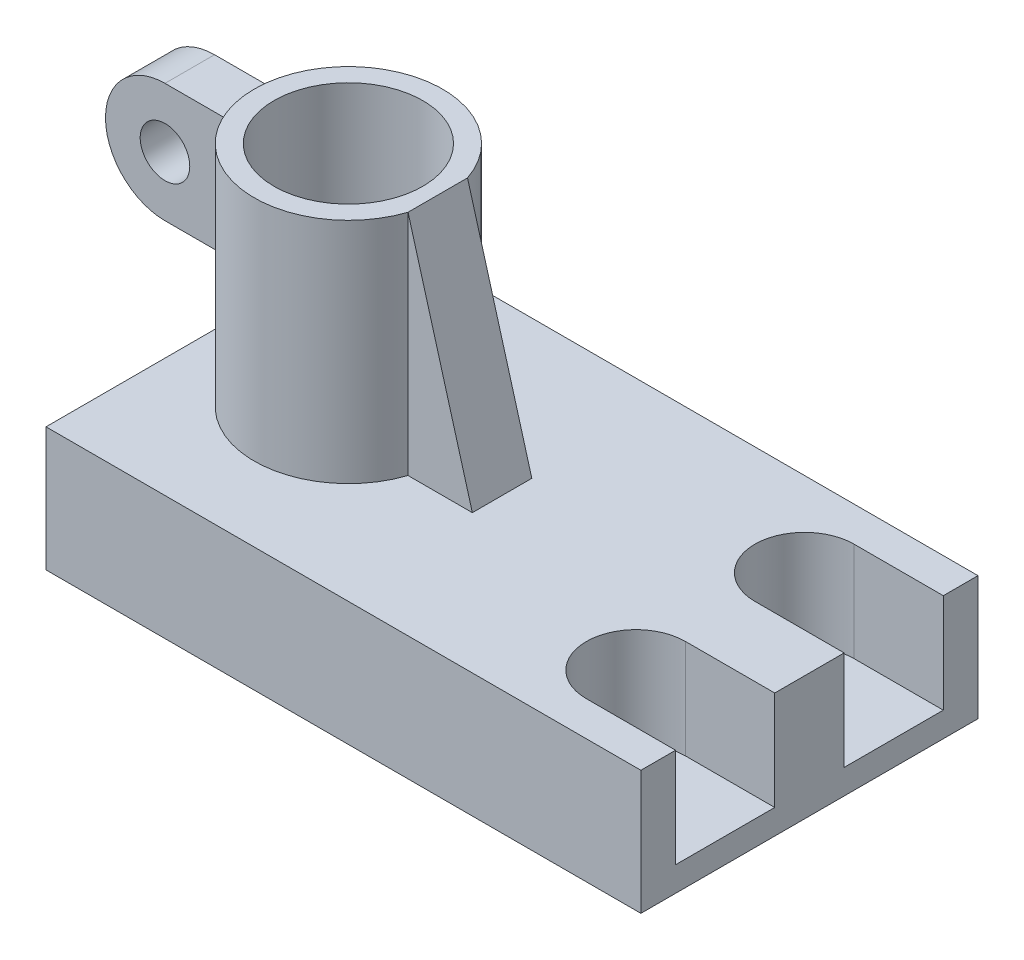
ISO-10303-21;
HEADER;
FILE_DESCRIPTION(('STEP AP214'),'2;1');
FILE_NAME('part.step','',(''),(''),'','','');
FILE_SCHEMA(('AUTOMOTIVE_DESIGN { 1 0 10303 214 1 1 1 1 }'));
ENDSEC;
DATA;
#1=APPLICATION_CONTEXT('core data for automotive mechanical design processes');
#2=APPLICATION_PROTOCOL_DEFINITION('international standard','automotive_design',2000,#1);
#3=PRODUCT_CONTEXT('',#1,'mechanical');
#4=PRODUCT('Part','Part','',(#3));
#5=PRODUCT_RELATED_PRODUCT_CATEGORY('part','',(#4));
#6=PRODUCT_DEFINITION_FORMATION('','',#4);
#7=PRODUCT_DEFINITION_CONTEXT('part definition',#1,'design');
#8=PRODUCT_DEFINITION('design','',#6,#7);
#9=PRODUCT_DEFINITION_SHAPE('','',#8);
#10=(LENGTH_UNIT() NAMED_UNIT(*) SI_UNIT(.MILLI.,.METRE.));
#11=(NAMED_UNIT(*) PLANE_ANGLE_UNIT() SI_UNIT($,.RADIAN.));
#12=(NAMED_UNIT(*) SI_UNIT($,.STERADIAN.) SOLID_ANGLE_UNIT());
#13=UNCERTAINTY_MEASURE_WITH_UNIT(LENGTH_MEASURE(1.E-05),#10,'distance_accuracy_value','');
#14=(GEOMETRIC_REPRESENTATION_CONTEXT(3) GLOBAL_UNCERTAINTY_ASSIGNED_CONTEXT((#13)) GLOBAL_UNIT_ASSIGNED_CONTEXT((#10,
#11,#12)) REPRESENTATION_CONTEXT('',''));
#15=CARTESIAN_POINT('',(0.,0.,0.));
#16=DIRECTION('',(0.,0.,1.));
#17=DIRECTION('',(1.,0.,0.));
#18=AXIS2_PLACEMENT_3D('',#15,#16,#17);
#19=CARTESIAN_POINT('',(60.,25.,34.));
#20=DIRECTION('',(-1.,0.,0.));
#21=DIRECTION('',(0.,0.,1.));
#22=AXIS2_PLACEMENT_3D('',#19,#20,#21);
#23=PLANE('',#22);
#24=DIRECTION('',(0.,0.,-1.));
#25=VECTOR('',#24,1.);
#26=CARTESIAN_POINT('',(60.,25.,34.));
#27=LINE('',#26,#25);
#28=CARTESIAN_POINT('',(60.,25.,7.));
#29=VERTEX_POINT('',#28);
#30=CARTESIAN_POINT('',(60.,25.,-7.));
#31=VERTEX_POINT('',#30);
#32=EDGE_CURVE('E216',#29,#31,#27,.T.);
#33=ORIENTED_EDGE('',*,*,#32,.F.);
#34=DIRECTION('',(0.,1.,0.));
#35=VECTOR('',#34,1.);
#36=CARTESIAN_POINT('',(60.,5.,7.));
#37=LINE('',#36,#35);
#38=CARTESIAN_POINT('',(60.,5.,7.));
#39=VERTEX_POINT('',#38);
#40=EDGE_CURVE('E329',#39,#29,#37,.T.);
#41=ORIENTED_EDGE('',*,*,#40,.F.);
#42=DIRECTION('',(0.,0.,-1.));
#43=VECTOR('',#42,1.);
#44=CARTESIAN_POINT('',(60.,5.,7.));
#45=LINE('',#44,#43);
#46=CARTESIAN_POINT('',(60.,5.,27.));
#47=VERTEX_POINT('',#46);
#48=EDGE_CURVE('E356',#47,#39,#45,.T.);
#49=ORIENTED_EDGE('',*,*,#48,.F.);
#50=DIRECTION('',(0.,1.,0.));
#51=VECTOR('',#50,1.);
#52=CARTESIAN_POINT('',(60.,5.,27.));
#53=LINE('',#52,#51);
#54=CARTESIAN_POINT('',(60.,25.,27.));
#55=VERTEX_POINT('',#54);
#56=EDGE_CURVE('E357',#47,#55,#53,.T.);
#57=ORIENTED_EDGE('',*,*,#56,.T.);
#58=CARTESIAN_POINT('',(60.,25.,34.));
#59=VERTEX_POINT('',#58);
#60=EDGE_CURVE('E213',#59,#55,#27,.T.);
#61=ORIENTED_EDGE('',*,*,#60,.F.);
#62=DIRECTION('',(0.,-1.,0.));
#63=VECTOR('',#62,1.);
#64=CARTESIAN_POINT('',(60.,25.,34.));
#65=LINE('',#64,#63);
#66=CARTESIAN_POINT('',(60.,0.,34.));
#67=VERTEX_POINT('',#66);
#68=EDGE_CURVE('E224',#59,#67,#65,.T.);
#69=ORIENTED_EDGE('',*,*,#68,.T.);
#70=DIRECTION('',(0.,0.,-1.));
#71=VECTOR('',#70,1.);
#72=CARTESIAN_POINT('',(60.,0.,34.));
#73=LINE('',#72,#71);
#74=CARTESIAN_POINT('',(60.,0.,-34.));
#75=VERTEX_POINT('',#74);
#76=EDGE_CURVE('E202',#67,#75,#73,.T.);
#77=ORIENTED_EDGE('',*,*,#76,.T.);
#78=DIRECTION('',(0.,-1.,0.));
#79=VECTOR('',#78,1.);
#80=CARTESIAN_POINT('',(60.,25.,-34.));
#81=LINE('',#80,#79);
#82=CARTESIAN_POINT('',(60.,25.,-34.));
#83=VERTEX_POINT('',#82);
#84=EDGE_CURVE('E239',#83,#75,#81,.T.);
#85=ORIENTED_EDGE('',*,*,#84,.F.);
#86=CARTESIAN_POINT('',(60.,25.,-27.));
#87=VERTEX_POINT('',#86);
#88=EDGE_CURVE('E218',#87,#83,#27,.T.);
#89=ORIENTED_EDGE('',*,*,#88,.F.);
#90=DIRECTION('',(0.,1.,0.));
#91=VECTOR('',#90,1.);
#92=CARTESIAN_POINT('',(60.,5.,-27.));
#93=LINE('',#92,#91);
#94=CARTESIAN_POINT('',(60.,5.,-27.));
#95=VERTEX_POINT('',#94);
#96=EDGE_CURVE('E386',#95,#87,#93,.T.);
#97=ORIENTED_EDGE('',*,*,#96,.F.);
#98=DIRECTION('',(0.,0.,-1.));
#99=VECTOR('',#98,1.);
#100=CARTESIAN_POINT('',(60.,5.,-27.));
#101=LINE('',#100,#99);
#102=CARTESIAN_POINT('',(60.,5.,-7.));
#103=VERTEX_POINT('',#102);
#104=EDGE_CURVE('E376',#103,#95,#101,.T.);
#105=ORIENTED_EDGE('',*,*,#104,.F.);
#106=DIRECTION('',(0.,1.,0.));
#107=VECTOR('',#106,1.);
#108=CARTESIAN_POINT('',(60.,5.,-7.));
#109=LINE('',#108,#107);
#110=EDGE_CURVE('E328',#103,#31,#109,.T.);
#111=ORIENTED_EDGE('',*,*,#110,.T.);
#112=EDGE_LOOP('',(#33,#41,#49,#57,#61,#69,#77,#85,#89,#97,#105,#111));
#113=FACE_BOUND('',#112,.T.);
#114=ADVANCED_FACE('F44',(#113),#23,.F.);
#115=CARTESIAN_POINT('',(-60.,25.,-34.));
#116=DIRECTION('',(0.,0.,1.));
#117=DIRECTION('',(1.,0.,0.));
#118=AXIS2_PLACEMENT_3D('',#115,#116,#117);
#119=PLANE('',#118);
#120=DIRECTION('',(-1.,0.,0.));
#121=VECTOR('',#120,1.);
#122=CARTESIAN_POINT('',(-60.,0.,-34.));
#123=LINE('',#122,#121);
#124=CARTESIAN_POINT('',(-60.,0.,-34.));
#125=VERTEX_POINT('',#124);
#126=EDGE_CURVE('E206',#75,#125,#123,.T.);
#127=ORIENTED_EDGE('',*,*,#126,.T.);
#128=DIRECTION('',(0.,-1.,0.));
#129=VECTOR('',#128,1.);
#130=CARTESIAN_POINT('',(-60.,25.,-34.));
#131=LINE('',#130,#129);
#132=CARTESIAN_POINT('',(-60.,25.,-34.));
#133=VERTEX_POINT('',#132);
#134=EDGE_CURVE('E240',#133,#125,#131,.T.);
#135=ORIENTED_EDGE('',*,*,#134,.F.);
#136=DIRECTION('',(-1.,0.,0.));
#137=VECTOR('',#136,1.);
#138=CARTESIAN_POINT('',(-60.,25.,-34.));
#139=LINE('',#138,#137);
#140=EDGE_CURVE('E219',#83,#133,#139,.T.);
#141=ORIENTED_EDGE('',*,*,#140,.F.);
#142=ORIENTED_EDGE('',*,*,#84,.T.);
#143=EDGE_LOOP('',(#127,#135,#141,#142));
#144=FACE_BOUND('',#143,.T.);
#145=ADVANCED_FACE('F313',(#144),#119,.F.);
#146=CARTESIAN_POINT('',(-60.,25.,34.));
#147=DIRECTION('',(1.,0.,0.));
#148=DIRECTION('',(0.,0.,-1.));
#149=AXIS2_PLACEMENT_3D('',#146,#147,#148);
#150=PLANE('',#149);
#151=DIRECTION('',(0.,0.,1.));
#152=VECTOR('',#151,1.);
#153=CARTESIAN_POINT('',(-60.,0.,34.));
#154=LINE('',#153,#152);
#155=CARTESIAN_POINT('',(-60.,0.,34.));
#156=VERTEX_POINT('',#155);
#157=EDGE_CURVE('E226',#125,#156,#154,.T.);
#158=ORIENTED_EDGE('',*,*,#157,.T.);
#159=DIRECTION('',(0.,-1.,0.));
#160=VECTOR('',#159,1.);
#161=CARTESIAN_POINT('',(-60.,25.,34.));
#162=LINE('',#161,#160);
#163=CARTESIAN_POINT('',(-60.,25.,34.));
#164=VERTEX_POINT('',#163);
#165=EDGE_CURVE('E234',#164,#156,#162,.T.);
#166=ORIENTED_EDGE('',*,*,#165,.F.);
#167=DIRECTION('',(0.,0.,1.));
#168=VECTOR('',#167,1.);
#169=CARTESIAN_POINT('',(-60.,25.,34.));
#170=LINE('',#169,#168);
#171=EDGE_CURVE('E225',#133,#164,#170,.T.);
#172=ORIENTED_EDGE('',*,*,#171,.F.);
#173=ORIENTED_EDGE('',*,*,#134,.T.);
#174=EDGE_LOOP('',(#158,#166,#172,#173));
#175=FACE_BOUND('',#174,.T.);
#176=ADVANCED_FACE('F322',(#175),#150,.F.);
#177=CARTESIAN_POINT('',(-60.,25.,34.));
#178=DIRECTION('',(0.,0.,-1.));
#179=DIRECTION('',(-1.,0.,0.));
#180=AXIS2_PLACEMENT_3D('',#177,#178,#179);
#181=PLANE('',#180);
#182=DIRECTION('',(1.,0.,0.));
#183=VECTOR('',#182,1.);
#184=CARTESIAN_POINT('',(-60.,0.,34.));
#185=LINE('',#184,#183);
#186=EDGE_CURVE('E229',#156,#67,#185,.T.);
#187=ORIENTED_EDGE('',*,*,#186,.T.);
#188=ORIENTED_EDGE('',*,*,#68,.F.);
#189=DIRECTION('',(1.,0.,0.));
#190=VECTOR('',#189,1.);
#191=CARTESIAN_POINT('',(-60.,25.,34.));
#192=LINE('',#191,#190);
#193=EDGE_CURVE('E222',#164,#59,#192,.T.);
#194=ORIENTED_EDGE('',*,*,#193,.F.);
#195=ORIENTED_EDGE('',*,*,#165,.T.);
#196=EDGE_LOOP('',(#187,#188,#194,#195));
#197=FACE_BOUND('',#196,.T.);
#198=ADVANCED_FACE('F354',(#197),#181,.F.);
#199=CARTESIAN_POINT('',(0.,25.,0.));
#200=DIRECTION('',(0.,-1.,0.));
#201=DIRECTION('',(0.,0.,-1.));
#202=AXIS2_PLACEMENT_3D('',#199,#200,#201);
#203=PLANE('',#202);
#204=CARTESIAN_POINT('',(-33.,25.,0.));
#205=DIRECTION('',(0.,-1.,0.));
#206=DIRECTION('',(0.,0.,-1.));
#207=AXIS2_PLACEMENT_3D('',#204,#205,#206);
#208=CIRCLE('',#207,19.);
#209=CARTESIAN_POINT('',(-14.9722436226801,25.,-6.));
#210=VERTEX_POINT('',#209);
#211=CARTESIAN_POINT('',(-14.9722436226801,25.,6.));
#212=VERTEX_POINT('',#211);
#213=EDGE_CURVE('E196',#210,#212,#208,.F.);
#214=ORIENTED_EDGE('',*,*,#213,.F.);
#215=DIRECTION('',(1.,0.,0.));
#216=VECTOR('',#215,1.);
#217=CARTESIAN_POINT('',(-77.002,25.,-6.));
#218=LINE('',#217,#216);
#219=CARTESIAN_POINT('',(-2.,25.,-6.));
#220=VERTEX_POINT('',#219);
#221=EDGE_CURVE('E430',#210,#220,#218,.T.);
#222=ORIENTED_EDGE('',*,*,#221,.T.);
#223=DIRECTION('',(0.,0.,-1.));
#224=VECTOR('',#223,1.);
#225=CARTESIAN_POINT('',(-2.,25.,6.));
#226=LINE('',#225,#224);
#227=CARTESIAN_POINT('',(-2.,25.,6.));
#228=VERTEX_POINT('',#227);
#229=EDGE_CURVE('E421',#228,#220,#226,.T.);
#230=ORIENTED_EDGE('',*,*,#229,.F.);
#231=DIRECTION('',(1.,0.,0.));
#232=VECTOR('',#231,1.);
#233=CARTESIAN_POINT('',(-77.002,25.,6.));
#234=LINE('',#233,#232);
#235=EDGE_CURVE('E186',#212,#228,#234,.T.);
#236=ORIENTED_EDGE('',*,*,#235,.F.);
#237=EDGE_LOOP('',(#214,#222,#230,#236));
#238=FACE_BOUND('',#237,.T.);
#239=CARTESIAN_POINT('',(42.,25.,17.));
#240=DIRECTION('',(0.,1.,0.));
#241=DIRECTION('',(0.,0.,1.));
#242=AXIS2_PLACEMENT_3D('',#239,#240,#241);
#243=CIRCLE('',#242,10.);
#244=CARTESIAN_POINT('',(42.,25.,7.));
#245=VERTEX_POINT('',#244);
#246=CARTESIAN_POINT('',(42.,25.,27.));
#247=VERTEX_POINT('',#246);
#248=EDGE_CURVE('E56',#245,#247,#243,.T.);
#249=ORIENTED_EDGE('',*,*,#248,.F.);
#250=DIRECTION('',(-1.,0.,0.));
#251=VECTOR('',#250,1.);
#252=CARTESIAN_POINT('',(42.,25.,7.));
#253=LINE('',#252,#251);
#254=EDGE_CURVE('E402',#29,#245,#253,.T.);
#255=ORIENTED_EDGE('',*,*,#254,.F.);
#256=ORIENTED_EDGE('',*,*,#32,.T.);
#257=DIRECTION('',(1.,0.,0.));
#258=VECTOR('',#257,1.);
#259=CARTESIAN_POINT('',(60.,25.,-7.));
#260=LINE('',#259,#258);
#261=CARTESIAN_POINT('',(42.,25.,-7.));
#262=VERTEX_POINT('',#261);
#263=EDGE_CURVE('E384',#262,#31,#260,.T.);
#264=ORIENTED_EDGE('',*,*,#263,.F.);
#265=CARTESIAN_POINT('',(42.,25.,-17.));
#266=DIRECTION('',(0.,1.,0.));
#267=DIRECTION('',(0.,0.,1.));
#268=AXIS2_PLACEMENT_3D('',#265,#266,#267);
#269=CIRCLE('',#268,10.);
#270=CARTESIAN_POINT('',(42.,25.,-27.));
#271=VERTEX_POINT('',#270);
#272=EDGE_CURVE('E70',#271,#262,#269,.T.);
#273=ORIENTED_EDGE('',*,*,#272,.F.);
#274=DIRECTION('',(-1.,0.,0.));
#275=VECTOR('',#274,1.);
#276=CARTESIAN_POINT('',(42.,25.,-27.));
#277=LINE('',#276,#275);
#278=EDGE_CURVE('E338',#87,#271,#277,.T.);
#279=ORIENTED_EDGE('',*,*,#278,.F.);
#280=ORIENTED_EDGE('',*,*,#88,.T.);
#281=ORIENTED_EDGE('',*,*,#140,.T.);
#282=ORIENTED_EDGE('',*,*,#171,.T.);
#283=ORIENTED_EDGE('',*,*,#193,.T.);
#284=ORIENTED_EDGE('',*,*,#60,.T.);
#285=DIRECTION('',(1.,0.,0.));
#286=VECTOR('',#285,1.);
#287=CARTESIAN_POINT('',(60.,25.,27.));
#288=LINE('',#287,#286);
#289=EDGE_CURVE('E404',#247,#55,#288,.T.);
#290=ORIENTED_EDGE('',*,*,#289,.F.);
#291=EDGE_LOOP('',(#249,#255,#256,#264,#273,#279,#280,#281,#282,#283,#284,#290));
#292=FACE_BOUND('',#291,.T.);
#293=ADVANCED_FACE('F340',(#238,#292),#203,.F.);
#294=CARTESIAN_POINT('',(0.,0.,0.));
#295=DIRECTION('',(0.,-1.,0.));
#296=DIRECTION('',(0.,0.,-1.));
#297=AXIS2_PLACEMENT_3D('',#294,#295,#296);
#298=PLANE('',#297);
#299=CARTESIAN_POINT('',(42.,0.,-17.));
#300=DIRECTION('',(0.,-1.,0.));
#301=DIRECTION('',(0.,0.,-1.));
#302=AXIS2_PLACEMENT_3D('',#299,#300,#301);
#303=CIRCLE('',#302,4.00000000000001);
#304=CARTESIAN_POINT('',(42.,0.,-21.));
#305=VERTEX_POINT('',#304);
#306=EDGE_CURVE('E381',#305,#305,#303,.T.);
#307=ORIENTED_EDGE('',*,*,#306,.F.);
#308=EDGE_LOOP('',(#307));
#309=FACE_BOUND('',#308,.T.);
#310=CARTESIAN_POINT('',(42.,0.,17.));
#311=DIRECTION('',(0.,-1.,0.));
#312=DIRECTION('',(0.,0.,-1.));
#313=AXIS2_PLACEMENT_3D('',#310,#311,#312);
#314=CIRCLE('',#313,4.00000000000001);
#315=CARTESIAN_POINT('',(42.,0.,13.));
#316=VERTEX_POINT('',#315);
#317=EDGE_CURVE('E416',#316,#316,#314,.T.);
#318=ORIENTED_EDGE('',*,*,#317,.F.);
#319=EDGE_LOOP('',(#318));
#320=FACE_BOUND('',#319,.T.);
#321=CARTESIAN_POINT('',(-33.,0.,0.));
#322=DIRECTION('',(0.,1.,0.));
#323=DIRECTION('',(0.,0.,1.));
#324=AXIS2_PLACEMENT_3D('',#321,#322,#323);
#325=CIRCLE('',#324,15.);
#326=CARTESIAN_POINT('',(-33.,0.,15.));
#327=VERTEX_POINT('',#326);
#328=EDGE_CURVE('E283',#327,#327,#325,.T.);
#329=ORIENTED_EDGE('',*,*,#328,.T.);
#330=EDGE_LOOP('',(#329));
#331=FACE_BOUND('',#330,.T.);
#332=ORIENTED_EDGE('',*,*,#76,.F.);
#333=ORIENTED_EDGE('',*,*,#186,.F.);
#334=ORIENTED_EDGE('',*,*,#157,.F.);
#335=ORIENTED_EDGE('',*,*,#126,.F.);
#336=EDGE_LOOP('',(#332,#333,#334,#335));
#337=FACE_BOUND('',#336,.T.);
#338=ADVANCED_FACE('F311',(#309,#320,#331,#337),#298,.T.);
#339=CARTESIAN_POINT('',(-33.,71.,0.));
#340=DIRECTION('',(0.,-1.,0.));
#341=DIRECTION('',(0.,0.,-1.));
#342=AXIS2_PLACEMENT_3D('',#339,#340,#341);
#343=CYLINDRICAL_SURFACE('',#342,19.);
#344=CARTESIAN_POINT('',(-33.,68.,0.));
#345=DIRECTION('',(0.,-1.,0.));
#346=DIRECTION('',(0.,0.,-1.));
#347=AXIS2_PLACEMENT_3D('',#344,#345,#346);
#348=CIRCLE('',#347,19.);
#349=CARTESIAN_POINT('',(-51.3303027798234,68.,5.));
#350=VERTEX_POINT('',#349);
#351=CARTESIAN_POINT('',(-51.3303027798234,68.,-5.));
#352=VERTEX_POINT('',#351);
#353=EDGE_CURVE('E250',#350,#352,#348,.T.);
#354=ORIENTED_EDGE('',*,*,#353,.F.);
#355=DIRECTION('',(0.,-1.,0.));
#356=VECTOR('',#355,1.);
#357=CARTESIAN_POINT('',(-51.3303027798234,71.,5.));
#358=LINE('',#357,#356);
#359=CARTESIAN_POINT('',(-51.3303027798234,44.,5.));
#360=VERTEX_POINT('',#359);
#361=EDGE_CURVE('E11',#350,#360,#358,.T.);
#362=ORIENTED_EDGE('',*,*,#361,.T.);
#363=CARTESIAN_POINT('',(-33.,44.,0.));
#364=DIRECTION('',(0.,1.,0.));
#365=DIRECTION('',(0.,0.,1.));
#366=AXIS2_PLACEMENT_3D('',#363,#364,#365);
#367=CIRCLE('',#366,19.);
#368=CARTESIAN_POINT('',(-51.3303027798234,44.,-5.));
#369=VERTEX_POINT('',#368);
#370=EDGE_CURVE('E55',#369,#360,#367,.T.);
#371=ORIENTED_EDGE('',*,*,#370,.F.);
#372=DIRECTION('',(0.,-1.,0.));
#373=VECTOR('',#372,1.);
#374=CARTESIAN_POINT('',(-51.3303027798234,71.,-5.));
#375=LINE('',#374,#373);
#376=EDGE_CURVE('E242',#352,#369,#375,.T.);
#377=ORIENTED_EDGE('',*,*,#376,.F.);
#378=EDGE_LOOP('',(#354,#362,#371,#377));
#379=FACE_BOUND('',#378,.T.);
#380=CARTESIAN_POINT('',(-33.,71.,0.));
#381=DIRECTION('',(0.,1.,0.));
#382=DIRECTION('',(0.,0.,1.));
#383=AXIS2_PLACEMENT_3D('',#380,#381,#382);
#384=CIRCLE('',#383,19.);
#385=CARTESIAN_POINT('',(-14.9722436226801,71.,-5.99999999999999));
#386=VERTEX_POINT('',#385);
#387=CARTESIAN_POINT('',(-14.9722436226801,71.,6.));
#388=VERTEX_POINT('',#387);
#389=EDGE_CURVE('E200',#386,#388,#384,.T.);
#390=ORIENTED_EDGE('',*,*,#389,.F.);
#391=DIRECTION('',(0.,-1.,0.));
#392=VECTOR('',#391,1.);
#393=CARTESIAN_POINT('',(-14.9722436226801,71.,-5.99999999999999));
#394=LINE('',#393,#392);
#395=EDGE_CURVE('E198',#210,#386,#394,.F.);
#396=ORIENTED_EDGE('',*,*,#395,.F.);
#397=ORIENTED_EDGE('',*,*,#213,.T.);
#398=DIRECTION('',(0.,-1.,0.));
#399=VECTOR('',#398,1.);
#400=CARTESIAN_POINT('',(-14.9722436226801,71.,6.00000000000001));
#401=LINE('',#400,#399);
#402=EDGE_CURVE('E190',#388,#212,#401,.T.);
#403=ORIENTED_EDGE('',*,*,#402,.F.);
#404=EDGE_LOOP('',(#390,#396,#397,#403));
#405=FACE_BOUND('',#404,.T.);
#406=ADVANCED_FACE('F193',(#379,#405),#343,.T.);
#407=CARTESIAN_POINT('',(-33.,71.,0.));
#408=DIRECTION('',(0.,1.,0.));
#409=DIRECTION('',(0.,0.,1.));
#410=AXIS2_PLACEMENT_3D('',#407,#408,#409);
#411=PLANE('',#410);
#412=DIRECTION('',(0.,0.,1.));
#413=VECTOR('',#412,1.);
#414=CARTESIAN_POINT('',(-14.9722436226801,71.,-14.));
#415=LINE('',#414,#413);
#416=EDGE_CURVE('E173',#386,#388,#415,.T.);
#417=ORIENTED_EDGE('',*,*,#416,.F.);
#418=ORIENTED_EDGE('',*,*,#389,.T.);
#419=EDGE_LOOP('',(#417,#418));
#420=FACE_BOUND('',#419,.T.);
#421=CARTESIAN_POINT('',(-33.,71.,0.));
#422=DIRECTION('',(0.,1.,0.));
#423=DIRECTION('',(0.,0.,1.));
#424=AXIS2_PLACEMENT_3D('',#421,#422,#423);
#425=CIRCLE('',#424,15.);
#426=CARTESIAN_POINT('',(-33.,71.,15.));
#427=VERTEX_POINT('',#426);
#428=EDGE_CURVE('E212',#427,#427,#425,.T.);
#429=ORIENTED_EDGE('',*,*,#428,.F.);
#430=EDGE_LOOP('',(#429));
#431=FACE_BOUND('',#430,.T.);
#432=ADVANCED_FACE('F205',(#420,#431),#411,.T.);
#433=CARTESIAN_POINT('',(-33.,38.,0.));
#434=DIRECTION('',(0.,1.,0.));
#435=DIRECTION('',(0.,0.,1.));
#436=AXIS2_PLACEMENT_3D('',#433,#434,#435);
#437=CYLINDRICAL_SURFACE('',#436,15.);
#438=CARTESIAN_POINT('',(-33.,38.,0.));
#439=DIRECTION('',(0.,1.,0.));
#440=DIRECTION('',(0.,0.,1.));
#441=AXIS2_PLACEMENT_3D('',#438,#439,#440);
#442=CIRCLE('',#441,15.);
#443=CARTESIAN_POINT('',(-33.,38.,15.));
#444=VERTEX_POINT('',#443);
#445=EDGE_CURVE('E204',#444,#444,#442,.T.);
#446=ORIENTED_EDGE('',*,*,#445,.F.);
#447=EDGE_LOOP('',(#446));
#448=FACE_BOUND('',#447,.T.);
#449=ORIENTED_EDGE('',*,*,#428,.T.);
#450=EDGE_LOOP('',(#449));
#451=FACE_BOUND('',#450,.T.);
#452=ADVANCED_FACE('F297',(#448,#451),#437,.F.);
#453=CARTESIAN_POINT('',(-33.,38.,0.));
#454=DIRECTION('',(0.,1.,0.));
#455=DIRECTION('',(0.,0.,1.));
#456=AXIS2_PLACEMENT_3D('',#453,#454,#455);
#457=PLANE('',#456);
#458=CARTESIAN_POINT('',(-33.,38.,0.));
#459=DIRECTION('',(0.,1.,0.));
#460=DIRECTION('',(0.,0.,1.));
#461=AXIS2_PLACEMENT_3D('',#458,#459,#460);
#462=CIRCLE('',#461,8.);
#463=CARTESIAN_POINT('',(-33.,38.,8.));
#464=VERTEX_POINT('',#463);
#465=EDGE_CURVE('E291',#464,#464,#462,.T.);
#466=ORIENTED_EDGE('',*,*,#465,.F.);
#467=EDGE_LOOP('',(#466));
#468=FACE_BOUND('',#467,.T.);
#469=ORIENTED_EDGE('',*,*,#445,.T.);
#470=EDGE_LOOP('',(#469));
#471=FACE_BOUND('',#470,.T.);
#472=ADVANCED_FACE('F308',(#468,#471),#457,.T.);
#473=CARTESIAN_POINT('',(-33.,33.,0.));
#474=DIRECTION('',(0.,1.,0.));
#475=DIRECTION('',(0.,0.,1.));
#476=AXIS2_PLACEMENT_3D('',#473,#474,#475);
#477=CYLINDRICAL_SURFACE('',#476,8.);
#478=CARTESIAN_POINT('',(-33.,33.,0.));
#479=DIRECTION('',(0.,1.,0.));
#480=DIRECTION('',(0.,0.,1.));
#481=AXIS2_PLACEMENT_3D('',#478,#479,#480);
#482=CIRCLE('',#481,8.);
#483=CARTESIAN_POINT('',(-33.,33.,8.));
#484=VERTEX_POINT('',#483);
#485=EDGE_CURVE('E288',#484,#484,#482,.T.);
#486=ORIENTED_EDGE('',*,*,#485,.F.);
#487=EDGE_LOOP('',(#486));
#488=FACE_BOUND('',#487,.T.);
#489=ORIENTED_EDGE('',*,*,#465,.T.);
#490=EDGE_LOOP('',(#489));
#491=FACE_BOUND('',#490,.T.);
#492=ADVANCED_FACE('F471',(#488,#491),#477,.F.);
#493=CARTESIAN_POINT('',(-33.,0.,0.));
#494=DIRECTION('',(0.,1.,0.));
#495=DIRECTION('',(0.,0.,1.));
#496=AXIS2_PLACEMENT_3D('',#493,#494,#495);
#497=CYLINDRICAL_SURFACE('',#496,15.);
#498=ORIENTED_EDGE('',*,*,#328,.F.);
#499=EDGE_LOOP('',(#498));
#500=FACE_BOUND('',#499,.T.);
#501=CARTESIAN_POINT('',(-33.,33.,0.));
#502=DIRECTION('',(0.,1.,0.));
#503=DIRECTION('',(0.,0.,1.));
#504=AXIS2_PLACEMENT_3D('',#501,#502,#503);
#505=CIRCLE('',#504,15.);
#506=CARTESIAN_POINT('',(-33.,33.,15.));
#507=VERTEX_POINT('',#506);
#508=EDGE_CURVE('E281',#507,#507,#505,.T.);
#509=ORIENTED_EDGE('',*,*,#508,.T.);
#510=EDGE_LOOP('',(#509));
#511=FACE_BOUND('',#510,.T.);
#512=ADVANCED_FACE('F482',(#500,#511),#497,.F.);
#513=CARTESIAN_POINT('',(-33.,33.,0.));
#514=DIRECTION('',(0.,1.,0.));
#515=DIRECTION('',(0.,0.,1.));
#516=AXIS2_PLACEMENT_3D('',#513,#514,#515);
#517=PLANE('',#516);
#518=ORIENTED_EDGE('',*,*,#485,.T.);
#519=EDGE_LOOP('',(#518));
#520=FACE_BOUND('',#519,.T.);
#521=ORIENTED_EDGE('',*,*,#508,.F.);
#522=EDGE_LOOP('',(#521));
#523=FACE_BOUND('',#522,.T.);
#524=ADVANCED_FACE('F500',(#520,#523),#517,.F.);
#525=CARTESIAN_POINT('',(-65.,56.,5.));
#526=DIRECTION('',(0.,0.,1.));
#527=DIRECTION('',(1.,0.,0.));
#528=AXIS2_PLACEMENT_3D('',#525,#526,#527);
#529=PLANE('',#528);
#530=CARTESIAN_POINT('',(-65.,56.,5.));
#531=DIRECTION('',(0.,0.,1.));
#532=DIRECTION('',(1.,0.,0.));
#533=AXIS2_PLACEMENT_3D('',#530,#531,#532);
#534=CIRCLE('',#533,5.);
#535=CARTESIAN_POINT('',(-60.,56.,5.));
#536=VERTEX_POINT('',#535);
#537=EDGE_CURVE('E391',#536,#536,#534,.T.);
#538=ORIENTED_EDGE('',*,*,#537,.F.);
#539=EDGE_LOOP('',(#538));
#540=FACE_BOUND('',#539,.T.);
#541=ORIENTED_EDGE('',*,*,#361,.F.);
#542=DIRECTION('',(-1.,0.,0.));
#543=VECTOR('',#542,1.);
#544=CARTESIAN_POINT('',(-65.,68.,5.));
#545=LINE('',#544,#543);
#546=CARTESIAN_POINT('',(-65.,68.,5.));
#547=VERTEX_POINT('',#546);
#548=EDGE_CURVE('E266',#350,#547,#545,.T.);
#549=ORIENTED_EDGE('',*,*,#548,.T.);
#550=CARTESIAN_POINT('',(-65.,56.,5.));
#551=DIRECTION('',(0.,0.,1.));
#552=DIRECTION('',(1.,0.,0.));
#553=AXIS2_PLACEMENT_3D('',#550,#551,#552);
#554=CIRCLE('',#553,12.);
#555=CARTESIAN_POINT('',(-65.,44.,5.));
#556=VERTEX_POINT('',#555);
#557=EDGE_CURVE('E261',#547,#556,#554,.T.);
#558=ORIENTED_EDGE('',*,*,#557,.T.);
#559=DIRECTION('',(1.,0.,0.));
#560=VECTOR('',#559,1.);
#561=CARTESIAN_POINT('',(-50.,44.,5.));
#562=LINE('',#561,#560);
#563=EDGE_CURVE('E253',#556,#360,#562,.T.);
#564=ORIENTED_EDGE('',*,*,#563,.T.);
#565=EDGE_LOOP('',(#541,#549,#558,#564));
#566=FACE_BOUND('',#565,.T.);
#567=ADVANCED_FACE('F262',(#540,#566),#529,.T.);
#568=CARTESIAN_POINT('',(-65.,56.,-5.));
#569=DIRECTION('',(0.,0.,1.));
#570=DIRECTION('',(1.,0.,0.));
#571=AXIS2_PLACEMENT_3D('',#568,#569,#570);
#572=PLANE('',#571);
#573=CARTESIAN_POINT('',(-65.,56.,-5.));
#574=DIRECTION('',(0.,0.,1.));
#575=DIRECTION('',(1.,0.,0.));
#576=AXIS2_PLACEMENT_3D('',#573,#574,#575);
#577=CIRCLE('',#576,5.);
#578=CARTESIAN_POINT('',(-60.,56.,-5.));
#579=VERTEX_POINT('',#578);
#580=EDGE_CURVE('E280',#579,#579,#577,.T.);
#581=ORIENTED_EDGE('',*,*,#580,.T.);
#582=EDGE_LOOP('',(#581));
#583=FACE_BOUND('',#582,.T.);
#584=DIRECTION('',(-1.,0.,0.));
#585=VECTOR('',#584,1.);
#586=CARTESIAN_POINT('',(-65.,68.,-5.));
#587=LINE('',#586,#585);
#588=CARTESIAN_POINT('',(-65.,68.,-5.));
#589=VERTEX_POINT('',#588);
#590=EDGE_CURVE('E269',#352,#589,#587,.T.);
#591=ORIENTED_EDGE('',*,*,#590,.F.);
#592=ORIENTED_EDGE('',*,*,#376,.T.);
#593=DIRECTION('',(1.,0.,0.));
#594=VECTOR('',#593,1.);
#595=CARTESIAN_POINT('',(-50.,44.,-5.));
#596=LINE('',#595,#594);
#597=CARTESIAN_POINT('',(-65.,44.,-5.));
#598=VERTEX_POINT('',#597);
#599=EDGE_CURVE('E260',#598,#369,#596,.T.);
#600=ORIENTED_EDGE('',*,*,#599,.F.);
#601=CARTESIAN_POINT('',(-65.,56.,-5.));
#602=DIRECTION('',(0.,0.,1.));
#603=DIRECTION('',(1.,0.,0.));
#604=AXIS2_PLACEMENT_3D('',#601,#602,#603);
#605=CIRCLE('',#604,12.);
#606=EDGE_CURVE('E274',#589,#598,#605,.T.);
#607=ORIENTED_EDGE('',*,*,#606,.F.);
#608=EDGE_LOOP('',(#591,#592,#600,#607));
#609=FACE_BOUND('',#608,.T.);
#610=ADVANCED_FACE('F516',(#583,#609),#572,.F.);
#611=CARTESIAN_POINT('',(-65.,56.,5.));
#612=DIRECTION('',(0.,0.,-1.));
#613=DIRECTION('',(-1.,0.,0.));
#614=AXIS2_PLACEMENT_3D('',#611,#612,#613);
#615=CYLINDRICAL_SURFACE('',#614,12.);
#616=ORIENTED_EDGE('',*,*,#606,.T.);
#617=DIRECTION('',(0.,0.,-1.));
#618=VECTOR('',#617,1.);
#619=CARTESIAN_POINT('',(-65.,44.,5.));
#620=LINE('',#619,#618);
#621=EDGE_CURVE('E285',#556,#598,#620,.T.);
#622=ORIENTED_EDGE('',*,*,#621,.F.);
#623=ORIENTED_EDGE('',*,*,#557,.F.);
#624=DIRECTION('',(0.,0.,-1.));
#625=VECTOR('',#624,1.);
#626=CARTESIAN_POINT('',(-65.,68.,5.));
#627=LINE('',#626,#625);
#628=EDGE_CURVE('E268',#547,#589,#627,.T.);
#629=ORIENTED_EDGE('',*,*,#628,.T.);
#630=EDGE_LOOP('',(#616,#622,#623,#629));
#631=FACE_BOUND('',#630,.T.);
#632=ADVANCED_FACE('F513',(#631),#615,.T.);
#633=CARTESIAN_POINT('',(-50.,44.,5.));
#634=DIRECTION('',(0.,1.,0.));
#635=DIRECTION('',(0.,0.,1.));
#636=AXIS2_PLACEMENT_3D('',#633,#634,#635);
#637=PLANE('',#636);
#638=ORIENTED_EDGE('',*,*,#599,.T.);
#639=ORIENTED_EDGE('',*,*,#370,.T.);
#640=ORIENTED_EDGE('',*,*,#563,.F.);
#641=ORIENTED_EDGE('',*,*,#621,.T.);
#642=EDGE_LOOP('',(#638,#639,#640,#641));
#643=FACE_BOUND('',#642,.T.);
#644=ADVANCED_FACE('F254',(#643),#637,.F.);
#645=CARTESIAN_POINT('',(-65.,68.,5.));
#646=DIRECTION('',(0.,-1.,0.));
#647=DIRECTION('',(0.,0.,-1.));
#648=AXIS2_PLACEMENT_3D('',#645,#646,#647);
#649=PLANE('',#648);
#650=ORIENTED_EDGE('',*,*,#548,.F.);
#651=ORIENTED_EDGE('',*,*,#353,.T.);
#652=ORIENTED_EDGE('',*,*,#590,.T.);
#653=ORIENTED_EDGE('',*,*,#628,.F.);
#654=EDGE_LOOP('',(#650,#651,#652,#653));
#655=FACE_BOUND('',#654,.T.);
#656=ADVANCED_FACE('F527',(#655),#649,.F.);
#657=CARTESIAN_POINT('',(-65.,56.,-5.));
#658=DIRECTION('',(0.,0.,1.));
#659=DIRECTION('',(1.,0.,0.));
#660=AXIS2_PLACEMENT_3D('',#657,#658,#659);
#661=CYLINDRICAL_SURFACE('',#660,5.);
#662=ORIENTED_EDGE('',*,*,#580,.F.);
#663=EDGE_LOOP('',(#662));
#664=FACE_BOUND('',#663,.T.);
#665=ORIENTED_EDGE('',*,*,#537,.T.);
#666=EDGE_LOOP('',(#665));
#667=FACE_BOUND('',#666,.T.);
#668=ADVANCED_FACE('F540',(#664,#667),#661,.F.);
#669=CARTESIAN_POINT('',(42.,5.,-17.));
#670=DIRECTION('',(0.,1.,0.));
#671=DIRECTION('',(0.,0.,1.));
#672=AXIS2_PLACEMENT_3D('',#669,#670,#671);
#673=CYLINDRICAL_SURFACE('',#672,10.);
#674=ORIENTED_EDGE('',*,*,#272,.T.);
#675=DIRECTION('',(0.,1.,0.));
#676=VECTOR('',#675,1.);
#677=CARTESIAN_POINT('',(42.,5.,-7.));
#678=LINE('',#677,#676);
#679=CARTESIAN_POINT('',(42.,5.,-7.));
#680=VERTEX_POINT('',#679);
#681=EDGE_CURVE('E382',#680,#262,#678,.T.);
#682=ORIENTED_EDGE('',*,*,#681,.F.);
#683=CARTESIAN_POINT('',(42.,5.,-17.));
#684=DIRECTION('',(0.,1.,0.));
#685=DIRECTION('',(0.,0.,1.));
#686=AXIS2_PLACEMENT_3D('',#683,#684,#685);
#687=CIRCLE('',#686,10.);
#688=CARTESIAN_POINT('',(42.,5.,-27.));
#689=VERTEX_POINT('',#688);
#690=EDGE_CURVE('E369',#689,#680,#687,.T.);
#691=ORIENTED_EDGE('',*,*,#690,.F.);
#692=DIRECTION('',(0.,1.,0.));
#693=VECTOR('',#692,1.);
#694=CARTESIAN_POINT('',(42.,5.,-27.));
#695=LINE('',#694,#693);
#696=EDGE_CURVE('E390',#689,#271,#695,.T.);
#697=ORIENTED_EDGE('',*,*,#696,.T.);
#698=EDGE_LOOP('',(#674,#682,#691,#697));
#699=FACE_BOUND('',#698,.T.);
#700=ADVANCED_FACE('F559',(#699),#673,.F.);
#701=CARTESIAN_POINT('',(42.,5.,-27.));
#702=DIRECTION('',(0.,0.,-1.));
#703=DIRECTION('',(-1.,0.,0.));
#704=AXIS2_PLACEMENT_3D('',#701,#702,#703);
#705=PLANE('',#704);
#706=ORIENTED_EDGE('',*,*,#278,.T.);
#707=ORIENTED_EDGE('',*,*,#696,.F.);
#708=DIRECTION('',(-1.,0.,0.));
#709=VECTOR('',#708,1.);
#710=CARTESIAN_POINT('',(42.,5.,-27.));
#711=LINE('',#710,#709);
#712=EDGE_CURVE('E377',#95,#689,#711,.T.);
#713=ORIENTED_EDGE('',*,*,#712,.F.);
#714=ORIENTED_EDGE('',*,*,#96,.T.);
#715=EDGE_LOOP('',(#706,#707,#713,#714));
#716=FACE_BOUND('',#715,.T.);
#717=ADVANCED_FACE('F574',(#716),#705,.F.);
#718=CARTESIAN_POINT('',(60.,5.,-7.));
#719=DIRECTION('',(0.,0.,1.));
#720=DIRECTION('',(1.,0.,0.));
#721=AXIS2_PLACEMENT_3D('',#718,#719,#720);
#722=PLANE('',#721);
#723=ORIENTED_EDGE('',*,*,#263,.T.);
#724=ORIENTED_EDGE('',*,*,#110,.F.);
#725=DIRECTION('',(1.,0.,0.));
#726=VECTOR('',#725,1.);
#727=CARTESIAN_POINT('',(60.,5.,-7.));
#728=LINE('',#727,#726);
#729=EDGE_CURVE('E373',#680,#103,#728,.T.);
#730=ORIENTED_EDGE('',*,*,#729,.F.);
#731=ORIENTED_EDGE('',*,*,#681,.T.);
#732=EDGE_LOOP('',(#723,#724,#730,#731));
#733=FACE_BOUND('',#732,.T.);
#734=ADVANCED_FACE('F584',(#733),#722,.F.);
#735=CARTESIAN_POINT('',(42.,5.,-17.));
#736=DIRECTION('',(0.,1.,0.));
#737=DIRECTION('',(0.,0.,1.));
#738=AXIS2_PLACEMENT_3D('',#735,#736,#737);
#739=PLANE('',#738);
#740=CARTESIAN_POINT('',(42.,5.,-17.));
#741=DIRECTION('',(0.,1.,0.));
#742=DIRECTION('',(0.,0.,1.));
#743=AXIS2_PLACEMENT_3D('',#740,#741,#742);
#744=CIRCLE('',#743,4.00000000000001);
#745=CARTESIAN_POINT('',(42.,5.,-13.));
#746=VERTEX_POINT('',#745);
#747=EDGE_CURVE('E417',#746,#746,#744,.T.);
#748=ORIENTED_EDGE('',*,*,#747,.F.);
#749=EDGE_LOOP('',(#748));
#750=FACE_BOUND('',#749,.T.);
#751=ORIENTED_EDGE('',*,*,#690,.T.);
#752=ORIENTED_EDGE('',*,*,#729,.T.);
#753=ORIENTED_EDGE('',*,*,#104,.T.);
#754=ORIENTED_EDGE('',*,*,#712,.T.);
#755=EDGE_LOOP('',(#751,#752,#753,#754));
#756=FACE_BOUND('',#755,.T.);
#757=ADVANCED_FACE('F593',(#750,#756),#739,.T.);
#758=CARTESIAN_POINT('',(42.,5.,17.));
#759=DIRECTION('',(0.,1.,0.));
#760=DIRECTION('',(0.,0.,1.));
#761=AXIS2_PLACEMENT_3D('',#758,#759,#760);
#762=CYLINDRICAL_SURFACE('',#761,10.);
#763=ORIENTED_EDGE('',*,*,#248,.T.);
#764=DIRECTION('',(0.,1.,0.));
#765=VECTOR('',#764,1.);
#766=CARTESIAN_POINT('',(42.,5.,27.));
#767=LINE('',#766,#765);
#768=CARTESIAN_POINT('',(42.,5.,27.));
#769=VERTEX_POINT('',#768);
#770=EDGE_CURVE('E365',#769,#247,#767,.T.);
#771=ORIENTED_EDGE('',*,*,#770,.F.);
#772=CARTESIAN_POINT('',(42.,5.,17.));
#773=DIRECTION('',(0.,1.,0.));
#774=DIRECTION('',(0.,0.,1.));
#775=AXIS2_PLACEMENT_3D('',#772,#773,#774);
#776=CIRCLE('',#775,10.);
#777=CARTESIAN_POINT('',(42.,5.,7.));
#778=VERTEX_POINT('',#777);
#779=EDGE_CURVE('E401',#778,#769,#776,.T.);
#780=ORIENTED_EDGE('',*,*,#779,.F.);
#781=DIRECTION('',(0.,1.,0.));
#782=VECTOR('',#781,1.);
#783=CARTESIAN_POINT('',(42.,5.,7.));
#784=LINE('',#783,#782);
#785=EDGE_CURVE('E364',#778,#245,#784,.T.);
#786=ORIENTED_EDGE('',*,*,#785,.T.);
#787=EDGE_LOOP('',(#763,#771,#780,#786));
#788=FACE_BOUND('',#787,.T.);
#789=ADVANCED_FACE('F601',(#788),#762,.F.);
#790=CARTESIAN_POINT('',(42.,5.,7.));
#791=DIRECTION('',(0.,0.,-1.));
#792=DIRECTION('',(-1.,0.,0.));
#793=AXIS2_PLACEMENT_3D('',#790,#791,#792);
#794=PLANE('',#793);
#795=ORIENTED_EDGE('',*,*,#254,.T.);
#796=ORIENTED_EDGE('',*,*,#785,.F.);
#797=DIRECTION('',(-1.,0.,0.));
#798=VECTOR('',#797,1.);
#799=CARTESIAN_POINT('',(42.,5.,7.));
#800=LINE('',#799,#798);
#801=EDGE_CURVE('E366',#39,#778,#800,.T.);
#802=ORIENTED_EDGE('',*,*,#801,.F.);
#803=ORIENTED_EDGE('',*,*,#40,.T.);
#804=EDGE_LOOP('',(#795,#796,#802,#803));
#805=FACE_BOUND('',#804,.T.);
#806=ADVANCED_FACE('F612',(#805),#794,.F.);
#807=CARTESIAN_POINT('',(60.,5.,27.));
#808=DIRECTION('',(0.,0.,1.));
#809=DIRECTION('',(1.,0.,0.));
#810=AXIS2_PLACEMENT_3D('',#807,#808,#809);
#811=PLANE('',#810);
#812=ORIENTED_EDGE('',*,*,#289,.T.);
#813=ORIENTED_EDGE('',*,*,#56,.F.);
#814=DIRECTION('',(1.,0.,0.));
#815=VECTOR('',#814,1.);
#816=CARTESIAN_POINT('',(60.,5.,27.));
#817=LINE('',#816,#815);
#818=EDGE_CURVE('E408',#769,#47,#817,.T.);
#819=ORIENTED_EDGE('',*,*,#818,.F.);
#820=ORIENTED_EDGE('',*,*,#770,.T.);
#821=EDGE_LOOP('',(#812,#813,#819,#820));
#822=FACE_BOUND('',#821,.T.);
#823=ADVANCED_FACE('F621',(#822),#811,.F.);
#824=CARTESIAN_POINT('',(42.,5.,17.));
#825=DIRECTION('',(0.,1.,0.));
#826=DIRECTION('',(0.,0.,1.));
#827=AXIS2_PLACEMENT_3D('',#824,#825,#826);
#828=PLANE('',#827);
#829=CARTESIAN_POINT('',(42.,5.,17.));
#830=DIRECTION('',(0.,1.,0.));
#831=DIRECTION('',(0.,0.,1.));
#832=AXIS2_PLACEMENT_3D('',#829,#830,#831);
#833=CIRCLE('',#832,4.00000000000001);
#834=CARTESIAN_POINT('',(42.,5.,21.));
#835=VERTEX_POINT('',#834);
#836=EDGE_CURVE('E419',#835,#835,#833,.T.);
#837=ORIENTED_EDGE('',*,*,#836,.F.);
#838=EDGE_LOOP('',(#837));
#839=FACE_BOUND('',#838,.T.);
#840=ORIENTED_EDGE('',*,*,#779,.T.);
#841=ORIENTED_EDGE('',*,*,#818,.T.);
#842=ORIENTED_EDGE('',*,*,#48,.T.);
#843=ORIENTED_EDGE('',*,*,#801,.T.);
#844=EDGE_LOOP('',(#840,#841,#842,#843));
#845=FACE_BOUND('',#844,.T.);
#846=ADVANCED_FACE('F633',(#839,#845),#828,.T.);
#847=CARTESIAN_POINT('',(42.,-15.,17.));
#848=DIRECTION('',(0.,1.,0.));
#849=DIRECTION('',(0.,0.,1.));
#850=AXIS2_PLACEMENT_3D('',#847,#848,#849);
#851=CYLINDRICAL_SURFACE('',#850,4.00000000000001);
#852=ORIENTED_EDGE('',*,*,#317,.T.);
#853=EDGE_LOOP('',(#852));
#854=FACE_BOUND('',#853,.T.);
#855=ORIENTED_EDGE('',*,*,#836,.T.);
#856=EDGE_LOOP('',(#855));
#857=FACE_BOUND('',#856,.T.);
#858=ADVANCED_FACE('F642',(#854,#857),#851,.F.);
#859=CARTESIAN_POINT('',(42.,-15.,-17.));
#860=DIRECTION('',(0.,1.,0.));
#861=DIRECTION('',(0.,0.,1.));
#862=AXIS2_PLACEMENT_3D('',#859,#860,#861);
#863=CYLINDRICAL_SURFACE('',#862,4.00000000000001);
#864=ORIENTED_EDGE('',*,*,#306,.T.);
#865=EDGE_LOOP('',(#864));
#866=FACE_BOUND('',#865,.T.);
#867=ORIENTED_EDGE('',*,*,#747,.T.);
#868=EDGE_LOOP('',(#867));
#869=FACE_BOUND('',#868,.T.);
#870=ADVANCED_FACE('F652',(#866,#869),#863,.F.);
#871=CARTESIAN_POINT('',(-77.002,71.,-5.99999999999999));
#872=DIRECTION('',(0.,0.,-1.));
#873=DIRECTION('',(0.,1.,0.));
#874=AXIS2_PLACEMENT_3D('',#871,#872,#873);
#875=PLANE('',#874);
#876=DIRECTION('',(-0.271419166644661,0.96246123868856,0.));
#877=VECTOR('',#876,1.);
#878=CARTESIAN_POINT('',(-19.5418742956856,87.2040597657867,-5.99999999999999));
#879=LINE('',#878,#877);
#880=EDGE_CURVE('E177',#220,#386,#879,.T.);
#881=ORIENTED_EDGE('',*,*,#880,.F.);
#882=ORIENTED_EDGE('',*,*,#221,.F.);
#883=ORIENTED_EDGE('',*,*,#395,.T.);
#884=EDGE_LOOP('',(#881,#882,#883));
#885=FACE_BOUND('',#884,.T.);
#886=ADVANCED_FACE('F433',(#885),#875,.T.);
#887=CARTESIAN_POINT('',(-77.002,71.,6.00000000000001));
#888=DIRECTION('',(0.,0.,1.));
#889=DIRECTION('',(0.,-1.,0.));
#890=AXIS2_PLACEMENT_3D('',#887,#888,#889);
#891=PLANE('',#890);
#892=DIRECTION('',(0.271419166644661,-0.96246123868856,0.));
#893=VECTOR('',#892,1.);
#894=CARTESIAN_POINT('',(-14.9722436226801,71.,6.));
#895=LINE('',#894,#893);
#896=EDGE_CURVE('E176',#388,#228,#895,.T.);
#897=ORIENTED_EDGE('',*,*,#896,.F.);
#898=ORIENTED_EDGE('',*,*,#402,.T.);
#899=ORIENTED_EDGE('',*,*,#235,.T.);
#900=EDGE_LOOP('',(#897,#898,#899));
#901=FACE_BOUND('',#900,.T.);
#902=ADVANCED_FACE('F187',(#901),#891,.T.);
#903=CARTESIAN_POINT('',(-14.9722436226801,71.,-14.));
#904=DIRECTION('',(-0.96246123868856,-0.271419166644661,0.));
#905=DIRECTION('',(0.271419166644661,-0.96246123868856,0.));
#906=AXIS2_PLACEMENT_3D('',#903,#904,#905);
#907=PLANE('',#906);
#908=ORIENTED_EDGE('',*,*,#880,.T.);
#909=ORIENTED_EDGE('',*,*,#416,.T.);
#910=ORIENTED_EDGE('',*,*,#896,.T.);
#911=ORIENTED_EDGE('',*,*,#229,.T.);
#912=EDGE_LOOP('',(#908,#909,#910,#911));
#913=FACE_BOUND('',#912,.T.);
#914=ADVANCED_FACE('F174',(#913),#907,.F.);
#915=CLOSED_SHELL('',(#114,#145,#176,#198,#293,#338,#406,#432,#452,#472,#492,#512,#524,#567,
#610,#632,#644,#656,#668,#700,#717,#734,#757,#789,#806,#823,#846,#858,#870,#886,#902,#914));
#916=MANIFOLD_SOLID_BREP('B2',#915);
#917=ADVANCED_BREP_SHAPE_REPRESENTATION('',(#18,#916),#14);
#918=SHAPE_DEFINITION_REPRESENTATION(#9,#917);
ENDSEC;
END-ISO-10303-21;
